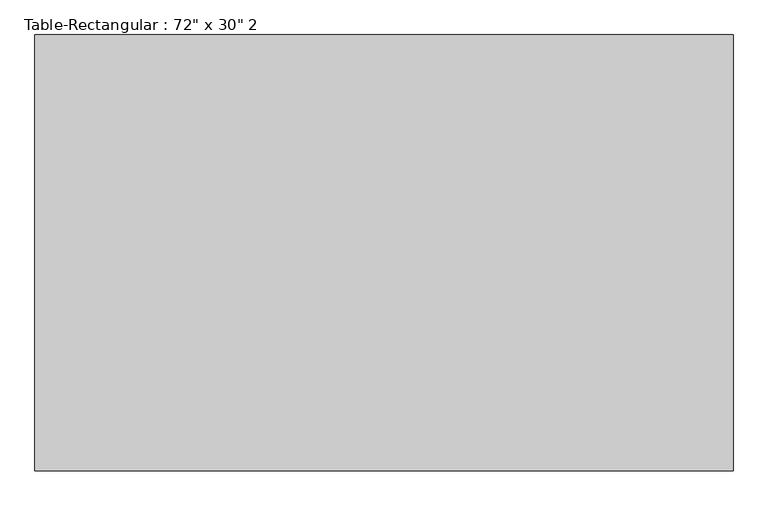
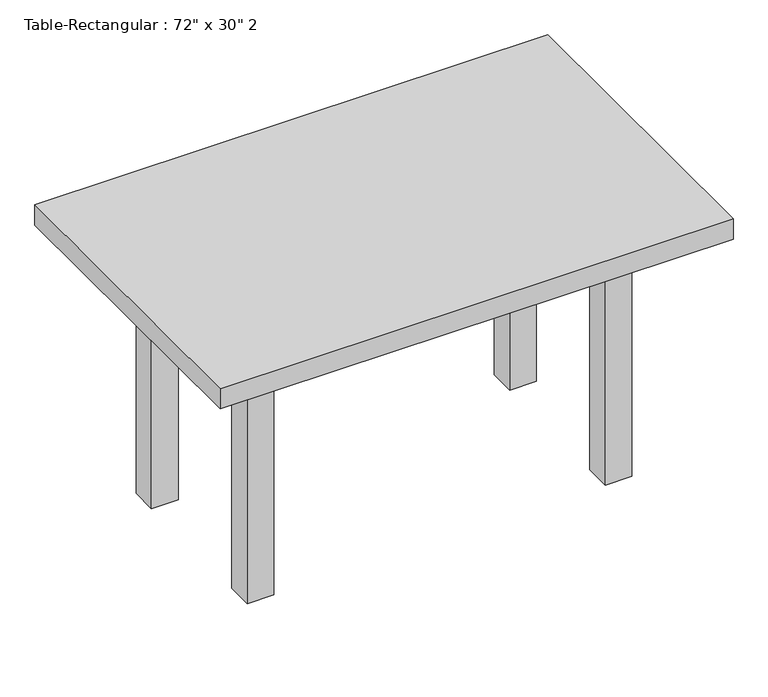
"""IFC4 building model written with IfcOpenShell, lengths in millimetres: furniture geometry."""

from ifc_helpers import new_model, si_unit, frame, origin, origin_with_axes, place, context, project, spatial, polyline, outline, extrude, source, transform, mapped, element, save


def furniture_d260d85f(model_context):
    return source(origin(), model_context, "Body", "SweptSolid", [
        extrude(outline(polyline([(393.7, 190.5), (393.7, 165.1), (-393.7, 165.1), (-393.7, 190.5), (393.7, 190.5)])), frame((0.0, 0.0, 533.4), z_axis=(0.0, 0.0, 1.0), x_axis=(1.0, 0.0, 0.0)), (0.0, 0.0, 1.0), 101.6),
        extrude(outline(polyline([(393.7, -190.5), (-393.7, -190.5), (-393.7, -165.1), (393.7, -165.1), (393.7, -190.5)])), frame((0.0, 0.0, 533.4), z_axis=(0.0, 0.0, 1.0), x_axis=(1.0, 0.0, 0.0)), (0.0, 0.0, 1.0), 101.6),
        extrude(outline(polyline([(-406.4, -165.1), (-431.8, -165.1), (-431.8, 165.1), (-406.4, 165.1), (-406.4, -165.1)])), frame((0.0, 0.0, 533.4), z_axis=(0.0, 0.0, 1.0), x_axis=(1.0, 0.0, 0.0)), (0.0, 0.0, 1.0), 101.6),
        extrude(outline(polyline([(406.4, -165.1), (406.4, 165.1), (431.8, 165.1), (431.8, -165.1), (406.4, -165.1)])), frame((0.0, 0.0, 533.4), z_axis=(0.0, 0.0, 1.0), x_axis=(1.0, 0.0, 0.0)), (0.0, 0.0, 1.0), 101.6),
        extrude(outline(polyline([(609.6, 381.0), (609.6, -381.0), (-609.6, -381.0), (-609.6, 381.0), (609.6, 381.0)])), frame((0.0, 0.0, 635.0), z_axis=(0.0, 0.0, 1.0), x_axis=(1.0, 0.0, 0.0)), (0.0, 0.0, 1.0), 50.8),
        extrude(outline(polyline([(-393.7, 228.6), (-393.7, 165.1), (-457.2, 165.1), (-457.2, 228.6), (-393.7, 228.6)])), origin_with_axes(), (0.0, 0.0, 1.0), 635.0),
        extrude(outline(polyline([(393.7, 228.6), (457.2, 228.6), (457.2, 165.1), (393.7, 165.1), (393.7, 228.6)])), origin_with_axes(), (0.0, 0.0, 1.0), 635.0),
        extrude(outline(polyline([(-393.7, -228.6), (-457.2, -228.6), (-457.2, -165.1), (-393.7, -165.1), (-393.7, -228.6)])), origin_with_axes(), (0.0, 0.0, 1.0), 635.0),
        extrude(outline(polyline([(393.7, -228.6), (393.7, -165.1), (457.2, -165.1), (457.2, -228.6), (393.7, -228.6)])), origin_with_axes(), (0.0, 0.0, 1.0), 635.0),
    ])


if __name__ == "__main__":
    model = new_model("IFC4")
    model_context = context("Model", 3, world=origin())
    ifc_project = project(units=[si_unit("LENGTHUNIT", "METRE", prefix="MILLI")], contexts=[model_context])
    site = spatial("IfcSite", under=ifc_project)
    building = spatial("IfcBuilding", under=site)
    placement = place(None, origin())
    furniture_shape = furniture_d260d85f(model_context)
    element("IfcFurniture", 1, ObjectType="Table-Rectangular : 72\" x 30\" 2", at=placement, inside=building, context=model_context, shape_type="MappedRepresentation", body=[
        mapped(furniture_shape, transform((0.0, 0.0, 0.0), x_axis=(1.0, 0.0, 0.0), y_axis=(0.0, 1.0, 0.0), z_axis=(0.0, 0.0, 1.0))),
    ])
    save(model, "model.ifc")

# Revit data of these elements
# Type "Table-Rectangular : 72\" x 30\" 2"
#   Assembly Code = "E2020200"
#   Height = 2' - 3"
#   Length = 4' - 0"
#   Width = 2' - 6"
#   Base Material = Birch
#   Top Material = Cherry
#   Default Elevation = 0
# Element 1 (IfcFurniture, "Table-Rectangular : 72\" x 30\" 2")
#   Materials on its faces: "Birch", "Cherry"
# Materials
#   "Birch": class "Wood", colour RGB 224 178 126, transparency 0, Description = "Betula Alleghaniensis", Cost = 0
#   "Cherry": class "Wood", colour RGB 226 177 128, transparency 0, Description = "Prunus Serotina", Cost = 0
